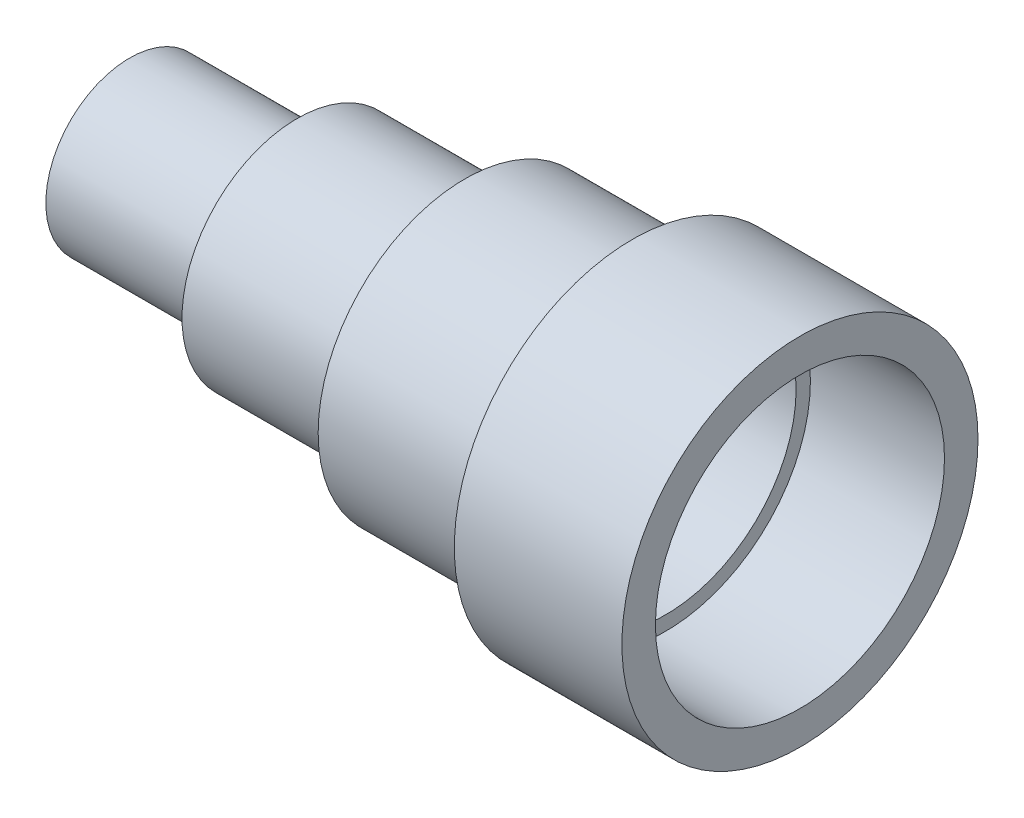
ISO-10303-21;
HEADER;
FILE_DESCRIPTION(('STEP AP214'),'2;1');
FILE_NAME('part.step','',(''),(''),'','','');
FILE_SCHEMA(('AUTOMOTIVE_DESIGN { 1 0 10303 214 1 1 1 1 }'));
ENDSEC;
DATA;
#1=APPLICATION_CONTEXT('core data for automotive mechanical design processes');
#2=APPLICATION_PROTOCOL_DEFINITION('international standard','automotive_design',2000,#1);
#3=PRODUCT_CONTEXT('',#1,'mechanical');
#4=PRODUCT('Part','Part','',(#3));
#5=PRODUCT_RELATED_PRODUCT_CATEGORY('part','',(#4));
#6=PRODUCT_DEFINITION_FORMATION('','',#4);
#7=PRODUCT_DEFINITION_CONTEXT('part definition',#1,'design');
#8=PRODUCT_DEFINITION('design','',#6,#7);
#9=PRODUCT_DEFINITION_SHAPE('','',#8);
#10=(LENGTH_UNIT() NAMED_UNIT(*) SI_UNIT(.MILLI.,.METRE.));
#11=(NAMED_UNIT(*) PLANE_ANGLE_UNIT() SI_UNIT($,.RADIAN.));
#12=(NAMED_UNIT(*) SI_UNIT($,.STERADIAN.) SOLID_ANGLE_UNIT());
#13=UNCERTAINTY_MEASURE_WITH_UNIT(LENGTH_MEASURE(1.E-05),#10,'distance_accuracy_value','');
#14=(GEOMETRIC_REPRESENTATION_CONTEXT(3) GLOBAL_UNCERTAINTY_ASSIGNED_CONTEXT((#13)) GLOBAL_UNIT_ASSIGNED_CONTEXT((#10,
#11,#12)) REPRESENTATION_CONTEXT('',''));
#15=CARTESIAN_POINT('',(0.,0.,0.));
#16=DIRECTION('',(0.,0.,1.));
#17=DIRECTION('',(1.,0.,0.));
#18=AXIS2_PLACEMENT_3D('',#15,#16,#17);
#19=CARTESIAN_POINT('',(40.,0.,-15.0355171036817));
#20=DIRECTION('',(1.,0.,0.));
#21=DIRECTION('',(0.,0.,-1.));
#22=AXIS2_PLACEMENT_3D('',#19,#20,#21);
#23=CYLINDRICAL_SURFACE('',#22,27.5);
#24=CARTESIAN_POINT('',(-40.,0.,-15.0355171036817));
#25=DIRECTION('',(1.,0.,0.));
#26=DIRECTION('',(0.,0.,-1.));
#27=AXIS2_PLACEMENT_3D('',#24,#25,#26);
#28=CIRCLE('',#27,27.5);
#29=CARTESIAN_POINT('',(-40.,0.,-42.5355171036817));
#30=VERTEX_POINT('',#29);
#31=EDGE_CURVE('E144',#30,#30,#28,.T.);
#32=ORIENTED_EDGE('',*,*,#31,.T.);
#33=EDGE_LOOP('',(#32));
#34=FACE_BOUND('',#33,.T.);
#35=CARTESIAN_POINT('',(0.,0.,-15.0355171036817));
#36=DIRECTION('',(1.,0.,0.));
#37=DIRECTION('',(0.,0.,-1.));
#38=AXIS2_PLACEMENT_3D('',#35,#36,#37);
#39=CIRCLE('',#38,27.5);
#40=CARTESIAN_POINT('',(0.,0.,-42.5355171036817));
#41=VERTEX_POINT('',#40);
#42=EDGE_CURVE('E102',#41,#41,#39,.T.);
#43=ORIENTED_EDGE('',*,*,#42,.F.);
#44=EDGE_LOOP('',(#43));
#45=FACE_BOUND('',#44,.T.);
#46=ADVANCED_FACE('F39',(#34,#45),#23,.T.);
#47=CARTESIAN_POINT('',(-40.,0.,-35.0355171036817));
#48=DIRECTION('',(-1.,0.,0.));
#49=DIRECTION('',(0.,0.,1.));
#50=AXIS2_PLACEMENT_3D('',#47,#48,#49);
#51=PLANE('',#50);
#52=CARTESIAN_POINT('',(-40.,0.,-15.0355171036817));
#53=DIRECTION('',(1.,0.,0.));
#54=DIRECTION('',(0.,0.,-1.));
#55=AXIS2_PLACEMENT_3D('',#52,#53,#54);
#56=CIRCLE('',#55,20.);
#57=CARTESIAN_POINT('',(-40.,0.,-35.0355171036817));
#58=VERTEX_POINT('',#57);
#59=EDGE_CURVE('E142',#58,#58,#56,.T.);
#60=ORIENTED_EDGE('',*,*,#59,.T.);
#61=EDGE_LOOP('',(#60));
#62=FACE_BOUND('',#61,.T.);
#63=ORIENTED_EDGE('',*,*,#31,.F.);
#64=EDGE_LOOP('',(#63));
#65=FACE_BOUND('',#64,.T.);
#66=ADVANCED_FACE('F175',(#62,#65),#51,.T.);
#67=CARTESIAN_POINT('',(40.,0.,-15.0355171036817));
#68=DIRECTION('',(1.,0.,0.));
#69=DIRECTION('',(0.,0.,-1.));
#70=AXIS2_PLACEMENT_3D('',#67,#68,#69);
#71=CYLINDRICAL_SURFACE('',#70,20.);
#72=CARTESIAN_POINT('',(-80.,0.,-15.0355171036817));
#73=DIRECTION('',(1.,0.,0.));
#74=DIRECTION('',(0.,0.,-1.));
#75=AXIS2_PLACEMENT_3D('',#72,#73,#74);
#76=CIRCLE('',#75,20.);
#77=CARTESIAN_POINT('',(-80.,0.,-35.0355171036817));
#78=VERTEX_POINT('',#77);
#79=EDGE_CURVE('E137',#78,#78,#76,.T.);
#80=ORIENTED_EDGE('',*,*,#79,.T.);
#81=EDGE_LOOP('',(#80));
#82=FACE_BOUND('',#81,.T.);
#83=ORIENTED_EDGE('',*,*,#59,.F.);
#84=EDGE_LOOP('',(#83));
#85=FACE_BOUND('',#84,.T.);
#86=ADVANCED_FACE('F176',(#82,#85),#71,.T.);
#87=CARTESIAN_POINT('',(-80.,0.,-15.0355171036817));
#88=DIRECTION('',(-1.,0.,0.));
#89=DIRECTION('',(0.,0.,1.));
#90=AXIS2_PLACEMENT_3D('',#87,#88,#89);
#91=PLANE('',#90);
#92=CARTESIAN_POINT('',(-80.,0.,-15.0355171036817));
#93=DIRECTION('',(-1.,0.,0.));
#94=DIRECTION('',(0.,0.,1.));
#95=AXIS2_PLACEMENT_3D('',#92,#93,#94);
#96=CIRCLE('',#95,15.);
#97=CARTESIAN_POINT('',(-80.,-14.6969384566991,-12.0355171036817));
#98=VERTEX_POINT('',#97);
#99=CARTESIAN_POINT('',(-80.,-14.6969384566991,-18.0355171036817));
#100=VERTEX_POINT('',#99);
#101=EDGE_CURVE('E52',#98,#100,#96,.T.);
#102=ORIENTED_EDGE('',*,*,#101,.F.);
#103=DIRECTION('',(0.,1.,0.));
#104=VECTOR('',#103,1.);
#105=CARTESIAN_POINT('',(-80.,-14.6969384566991,-12.0355171036817));
#106=LINE('',#105,#104);
#107=CARTESIAN_POINT('',(-80.,-18.,-12.0355171036817));
#108=VERTEX_POINT('',#107);
#109=EDGE_CURVE('E100',#108,#98,#106,.T.);
#110=ORIENTED_EDGE('',*,*,#109,.F.);
#111=DIRECTION('',(0.,0.,1.));
#112=VECTOR('',#111,1.);
#113=CARTESIAN_POINT('',(-80.,-18.,-15.0355171036817));
#114=LINE('',#113,#112);
#115=CARTESIAN_POINT('',(-80.,-18.,-18.0355171036817));
#116=VERTEX_POINT('',#115);
#117=EDGE_CURVE('E83',#116,#108,#114,.T.);
#118=ORIENTED_EDGE('',*,*,#117,.F.);
#119=DIRECTION('',(0.,-1.,0.));
#120=VECTOR('',#119,1.);
#121=CARTESIAN_POINT('',(-80.,-14.6969384566991,-18.0355171036817));
#122=LINE('',#121,#120);
#123=EDGE_CURVE('E89',#100,#116,#122,.T.);
#124=ORIENTED_EDGE('',*,*,#123,.F.);
#125=EDGE_LOOP('',(#102,#110,#118,#124));
#126=FACE_BOUND('',#125,.T.);
#127=ORIENTED_EDGE('',*,*,#79,.F.);
#128=EDGE_LOOP('',(#127));
#129=FACE_BOUND('',#128,.T.);
#130=ADVANCED_FACE('F94',(#126,#129),#91,.T.);
#131=CARTESIAN_POINT('',(-32.,0.,-40.273612341777));
#132=DIRECTION('',(1.,0.,0.));
#133=DIRECTION('',(0.,0.,-1.));
#134=AXIS2_PLACEMENT_3D('',#131,#132,#133);
#135=PLANE('',#134);
#136=CARTESIAN_POINT('',(-32.,0.,-15.0355171036817));
#137=DIRECTION('',(1.,0.,0.));
#138=DIRECTION('',(0.,0.,-1.));
#139=AXIS2_PLACEMENT_3D('',#136,#137,#138);
#140=CIRCLE('',#139,15.);
#141=CARTESIAN_POINT('',(-32.,-14.6969384566991,-18.0355171036817));
#142=VERTEX_POINT('',#141);
#143=CARTESIAN_POINT('',(-32.,-14.6969384566991,-12.0355171036817));
#144=VERTEX_POINT('',#143);
#145=EDGE_CURVE('E11',#142,#144,#140,.T.);
#146=ORIENTED_EDGE('',*,*,#145,.F.);
#147=DIRECTION('',(0.,1.,0.));
#148=VECTOR('',#147,1.);
#149=CARTESIAN_POINT('',(-32.,0.,-18.0355171036817));
#150=LINE('',#149,#148);
#151=CARTESIAN_POINT('',(-32.,-18.,-18.0355171036817));
#152=VERTEX_POINT('',#151);
#153=EDGE_CURVE('E146',#152,#142,#150,.T.);
#154=ORIENTED_EDGE('',*,*,#153,.F.);
#155=DIRECTION('',(0.,0.,-1.));
#156=VECTOR('',#155,1.);
#157=CARTESIAN_POINT('',(-32.,-18.,-40.273612341777));
#158=LINE('',#157,#156);
#159=CARTESIAN_POINT('',(-32.,-18.,-12.0355171036817));
#160=VERTEX_POINT('',#159);
#161=EDGE_CURVE('E82',#160,#152,#158,.T.);
#162=ORIENTED_EDGE('',*,*,#161,.F.);
#163=DIRECTION('',(0.,-1.,0.));
#164=VECTOR('',#163,1.);
#165=CARTESIAN_POINT('',(-32.,0.,-12.0355171036817));
#166=LINE('',#165,#164);
#167=EDGE_CURVE('E46',#144,#160,#166,.T.);
#168=ORIENTED_EDGE('',*,*,#167,.F.);
#169=EDGE_LOOP('',(#146,#154,#162,#168));
#170=FACE_BOUND('',#169,.T.);
#171=CARTESIAN_POINT('',(-32.,0.,-15.0355171036817));
#172=DIRECTION('',(1.,0.,0.));
#173=DIRECTION('',(0.,0.,-1.));
#174=AXIS2_PLACEMENT_3D('',#171,#172,#173);
#175=CIRCLE('',#174,25.2380952380952);
#176=CARTESIAN_POINT('',(-32.,0.,-40.273612341777));
#177=VERTEX_POINT('',#176);
#178=EDGE_CURVE('E138',#177,#177,#175,.T.);
#179=ORIENTED_EDGE('',*,*,#178,.T.);
#180=EDGE_LOOP('',(#179));
#181=FACE_BOUND('',#180,.T.);
#182=ADVANCED_FACE('F156',(#170,#181),#135,.T.);
#183=CARTESIAN_POINT('',(40.,0.,-15.0355171036817));
#184=DIRECTION('',(1.,0.,0.));
#185=DIRECTION('',(0.,0.,-1.));
#186=AXIS2_PLACEMENT_3D('',#183,#184,#185);
#187=CYLINDRICAL_SURFACE('',#186,25.2380952380952);
#188=CARTESIAN_POINT('',(8.00000000000001,0.,-15.0355171036817));
#189=DIRECTION('',(1.,0.,0.));
#190=DIRECTION('',(0.,0.,-1.));
#191=AXIS2_PLACEMENT_3D('',#188,#189,#190);
#192=CIRCLE('',#191,25.2380952380952);
#193=CARTESIAN_POINT('',(8.,0.,-40.273612341777));
#194=VERTEX_POINT('',#193);
#195=EDGE_CURVE('E135',#194,#194,#192,.T.);
#196=ORIENTED_EDGE('',*,*,#195,.T.);
#197=EDGE_LOOP('',(#196));
#198=FACE_BOUND('',#197,.T.);
#199=ORIENTED_EDGE('',*,*,#178,.F.);
#200=EDGE_LOOP('',(#199));
#201=FACE_BOUND('',#200,.T.);
#202=ADVANCED_FACE('F227',(#198,#201),#187,.F.);
#203=CARTESIAN_POINT('',(8.,0.,-46.1228186909833));
#204=DIRECTION('',(1.,0.,0.));
#205=DIRECTION('',(0.,0.,-1.));
#206=AXIS2_PLACEMENT_3D('',#203,#204,#205);
#207=PLANE('',#206);
#208=CARTESIAN_POINT('',(8.00000000000001,0.,-15.0355171036817));
#209=DIRECTION('',(1.,0.,0.));
#210=DIRECTION('',(0.,0.,-1.));
#211=AXIS2_PLACEMENT_3D('',#208,#209,#210);
#212=CIRCLE('',#211,31.0873015873016);
#213=CARTESIAN_POINT('',(8.00000000000001,0.,-46.1228186909833));
#214=VERTEX_POINT('',#213);
#215=EDGE_CURVE('E128',#214,#214,#212,.T.);
#216=ORIENTED_EDGE('',*,*,#215,.T.);
#217=EDGE_LOOP('',(#216));
#218=FACE_BOUND('',#217,.T.);
#219=ORIENTED_EDGE('',*,*,#195,.F.);
#220=EDGE_LOOP('',(#219));
#221=FACE_BOUND('',#220,.T.);
#222=ADVANCED_FACE('F221',(#218,#221),#207,.T.);
#223=CARTESIAN_POINT('',(40.,0.,-15.0355171036817));
#224=DIRECTION('',(1.,0.,0.));
#225=DIRECTION('',(0.,0.,-1.));
#226=AXIS2_PLACEMENT_3D('',#223,#224,#225);
#227=CYLINDRICAL_SURFACE('',#226,31.0873015873016);
#228=CARTESIAN_POINT('',(48.,0.,-15.0355171036817));
#229=DIRECTION('',(1.,0.,0.));
#230=DIRECTION('',(0.,0.,-1.));
#231=AXIS2_PLACEMENT_3D('',#228,#229,#230);
#232=CIRCLE('',#231,31.0873015873016);
#233=CARTESIAN_POINT('',(48.,0.,-46.1228186909833));
#234=VERTEX_POINT('',#233);
#235=EDGE_CURVE('E130',#234,#234,#232,.T.);
#236=ORIENTED_EDGE('',*,*,#235,.T.);
#237=EDGE_LOOP('',(#236));
#238=FACE_BOUND('',#237,.T.);
#239=ORIENTED_EDGE('',*,*,#215,.F.);
#240=EDGE_LOOP('',(#239));
#241=FACE_BOUND('',#240,.T.);
#242=ADVANCED_FACE('F217',(#238,#241),#227,.F.);
#243=CARTESIAN_POINT('',(48.,0.,-49.5355171036817));
#244=DIRECTION('',(1.,0.,0.));
#245=DIRECTION('',(0.,0.,-1.));
#246=AXIS2_PLACEMENT_3D('',#243,#244,#245);
#247=PLANE('',#246);
#248=CARTESIAN_POINT('',(48.,0.,-15.0355171036817));
#249=DIRECTION('',(1.,0.,0.));
#250=DIRECTION('',(0.,0.,-1.));
#251=AXIS2_PLACEMENT_3D('',#248,#249,#250);
#252=CIRCLE('',#251,34.5);
#253=CARTESIAN_POINT('',(48.,0.,-49.5355171036817));
#254=VERTEX_POINT('',#253);
#255=EDGE_CURVE('E122',#254,#254,#252,.T.);
#256=ORIENTED_EDGE('',*,*,#255,.T.);
#257=EDGE_LOOP('',(#256));
#258=FACE_BOUND('',#257,.T.);
#259=ORIENTED_EDGE('',*,*,#235,.F.);
#260=EDGE_LOOP('',(#259));
#261=FACE_BOUND('',#260,.T.);
#262=ADVANCED_FACE('F215',(#258,#261),#247,.T.);
#263=CARTESIAN_POINT('',(40.,0.,-15.0355171036817));
#264=DIRECTION('',(1.,0.,0.));
#265=DIRECTION('',(0.,0.,-1.));
#266=AXIS2_PLACEMENT_3D('',#263,#264,#265);
#267=CYLINDRICAL_SURFACE('',#266,34.5);
#268=CARTESIAN_POINT('',(80.,0.,-15.0355171036817));
#269=DIRECTION('',(1.,0.,0.));
#270=DIRECTION('',(0.,0.,-1.));
#271=AXIS2_PLACEMENT_3D('',#268,#269,#270);
#272=CIRCLE('',#271,34.5);
#273=CARTESIAN_POINT('',(80.,0.,-49.5355171036817));
#274=VERTEX_POINT('',#273);
#275=EDGE_CURVE('E123',#274,#274,#272,.T.);
#276=ORIENTED_EDGE('',*,*,#275,.T.);
#277=EDGE_LOOP('',(#276));
#278=FACE_BOUND('',#277,.T.);
#279=ORIENTED_EDGE('',*,*,#255,.F.);
#280=EDGE_LOOP('',(#279));
#281=FACE_BOUND('',#280,.T.);
#282=ADVANCED_FACE('F206',(#278,#281),#267,.F.);
#283=CARTESIAN_POINT('',(80.,0.,-57.5355171036817));
#284=DIRECTION('',(1.,0.,0.));
#285=DIRECTION('',(0.,0.,-1.));
#286=AXIS2_PLACEMENT_3D('',#283,#284,#285);
#287=PLANE('',#286);
#288=CARTESIAN_POINT('',(80.,0.,-15.0355171036817));
#289=DIRECTION('',(1.,0.,0.));
#290=DIRECTION('',(0.,0.,-1.));
#291=AXIS2_PLACEMENT_3D('',#288,#289,#290);
#292=CIRCLE('',#291,42.5);
#293=CARTESIAN_POINT('',(80.,0.,-57.5355171036817));
#294=VERTEX_POINT('',#293);
#295=EDGE_CURVE('E120',#294,#294,#292,.T.);
#296=ORIENTED_EDGE('',*,*,#295,.T.);
#297=EDGE_LOOP('',(#296));
#298=FACE_BOUND('',#297,.T.);
#299=ORIENTED_EDGE('',*,*,#275,.F.);
#300=EDGE_LOOP('',(#299));
#301=FACE_BOUND('',#300,.T.);
#302=ADVANCED_FACE('F199',(#298,#301),#287,.T.);
#303=CARTESIAN_POINT('',(40.,0.,-15.0355171036817));
#304=DIRECTION('',(1.,0.,0.));
#305=DIRECTION('',(0.,0.,-1.));
#306=AXIS2_PLACEMENT_3D('',#303,#304,#305);
#307=CYLINDRICAL_SURFACE('',#306,42.5);
#308=CARTESIAN_POINT('',(40.,0.,-15.0355171036817));
#309=DIRECTION('',(1.,0.,0.));
#310=DIRECTION('',(0.,0.,-1.));
#311=AXIS2_PLACEMENT_3D('',#308,#309,#310);
#312=CIRCLE('',#311,42.5);
#313=CARTESIAN_POINT('',(40.,0.,-57.5355171036817));
#314=VERTEX_POINT('',#313);
#315=EDGE_CURVE('E113',#314,#314,#312,.T.);
#316=ORIENTED_EDGE('',*,*,#315,.T.);
#317=EDGE_LOOP('',(#316));
#318=FACE_BOUND('',#317,.T.);
#319=ORIENTED_EDGE('',*,*,#295,.F.);
#320=EDGE_LOOP('',(#319));
#321=FACE_BOUND('',#320,.T.);
#322=ADVANCED_FACE('F192',(#318,#321),#307,.T.);
#323=CARTESIAN_POINT('',(40.,0.,-50.0355171036817));
#324=DIRECTION('',(-1.,0.,0.));
#325=DIRECTION('',(0.,0.,1.));
#326=AXIS2_PLACEMENT_3D('',#323,#324,#325);
#327=PLANE('',#326);
#328=CARTESIAN_POINT('',(40.,0.,-15.0355171036817));
#329=DIRECTION('',(1.,0.,0.));
#330=DIRECTION('',(0.,0.,-1.));
#331=AXIS2_PLACEMENT_3D('',#328,#329,#330);
#332=CIRCLE('',#331,35.);
#333=CARTESIAN_POINT('',(40.,0.,-50.0355171036817));
#334=VERTEX_POINT('',#333);
#335=EDGE_CURVE('E115',#334,#334,#332,.T.);
#336=ORIENTED_EDGE('',*,*,#335,.T.);
#337=EDGE_LOOP('',(#336));
#338=FACE_BOUND('',#337,.T.);
#339=ORIENTED_EDGE('',*,*,#315,.F.);
#340=EDGE_LOOP('',(#339));
#341=FACE_BOUND('',#340,.T.);
#342=ADVANCED_FACE('F190',(#338,#341),#327,.T.);
#343=CARTESIAN_POINT('',(40.,0.,-15.0355171036817));
#344=DIRECTION('',(1.,0.,0.));
#345=DIRECTION('',(0.,0.,-1.));
#346=AXIS2_PLACEMENT_3D('',#343,#344,#345);
#347=CYLINDRICAL_SURFACE('',#346,35.);
#348=CARTESIAN_POINT('',(0.,0.,-15.0355171036817));
#349=DIRECTION('',(1.,0.,0.));
#350=DIRECTION('',(0.,0.,-1.));
#351=AXIS2_PLACEMENT_3D('',#348,#349,#350);
#352=CIRCLE('',#351,35.);
#353=CARTESIAN_POINT('',(0.,0.,-50.0355171036817));
#354=VERTEX_POINT('',#353);
#355=EDGE_CURVE('E108',#354,#354,#352,.T.);
#356=ORIENTED_EDGE('',*,*,#355,.T.);
#357=EDGE_LOOP('',(#356));
#358=FACE_BOUND('',#357,.T.);
#359=ORIENTED_EDGE('',*,*,#335,.F.);
#360=EDGE_LOOP('',(#359));
#361=FACE_BOUND('',#360,.T.);
#362=ADVANCED_FACE('F169',(#358,#361),#347,.T.);
#363=CARTESIAN_POINT('',(0.,0.,-42.5355171036817));
#364=DIRECTION('',(-1.,0.,0.));
#365=DIRECTION('',(0.,0.,1.));
#366=AXIS2_PLACEMENT_3D('',#363,#364,#365);
#367=PLANE('',#366);
#368=ORIENTED_EDGE('',*,*,#42,.T.);
#369=EDGE_LOOP('',(#368));
#370=FACE_BOUND('',#369,.T.);
#371=ORIENTED_EDGE('',*,*,#355,.F.);
#372=EDGE_LOOP('',(#371));
#373=FACE_BOUND('',#372,.T.);
#374=ADVANCED_FACE('F159',(#370,#373),#367,.T.);
#375=CARTESIAN_POINT('',(80.,0.,-15.0355171036817));
#376=DIRECTION('',(-1.,0.,0.));
#377=DIRECTION('',(0.,0.,1.));
#378=AXIS2_PLACEMENT_3D('',#375,#376,#377);
#379=CYLINDRICAL_SURFACE('',#378,15.);
#380=ORIENTED_EDGE('',*,*,#145,.T.);
#381=DIRECTION('',(-1.,0.,0.));
#382=VECTOR('',#381,1.);
#383=CARTESIAN_POINT('',(80.,-14.6969384566991,-12.0355171036817));
#384=LINE('',#383,#382);
#385=EDGE_CURVE('E105',#144,#98,#384,.T.);
#386=ORIENTED_EDGE('',*,*,#385,.T.);
#387=ORIENTED_EDGE('',*,*,#101,.T.);
#388=DIRECTION('',(-1.,0.,0.));
#389=VECTOR('',#388,1.);
#390=CARTESIAN_POINT('',(80.,-14.6969384566991,-18.0355171036818));
#391=LINE('',#390,#389);
#392=EDGE_CURVE('E87',#142,#100,#391,.T.);
#393=ORIENTED_EDGE('',*,*,#392,.F.);
#394=EDGE_LOOP('',(#380,#386,#387,#393));
#395=FACE_BOUND('',#394,.T.);
#396=ADVANCED_FACE('F158',(#395),#379,.F.);
#397=CARTESIAN_POINT('',(80.,-14.6969384566991,-12.0355171036817));
#398=DIRECTION('',(0.,0.,1.));
#399=DIRECTION('',(1.,0.,0.));
#400=AXIS2_PLACEMENT_3D('',#397,#398,#399);
#401=PLANE('',#400);
#402=ORIENTED_EDGE('',*,*,#167,.T.);
#403=DIRECTION('',(-1.,0.,0.));
#404=VECTOR('',#403,1.);
#405=CARTESIAN_POINT('',(80.,-18.,-12.0355171036817));
#406=LINE('',#405,#404);
#407=EDGE_CURVE('E88',#160,#108,#406,.T.);
#408=ORIENTED_EDGE('',*,*,#407,.T.);
#409=ORIENTED_EDGE('',*,*,#109,.T.);
#410=ORIENTED_EDGE('',*,*,#385,.F.);
#411=EDGE_LOOP('',(#402,#408,#409,#410));
#412=FACE_BOUND('',#411,.T.);
#413=ADVANCED_FACE('F153',(#412),#401,.F.);
#414=CARTESIAN_POINT('',(80.,-18.,-15.0355171036817));
#415=DIRECTION('',(0.,-1.,0.));
#416=DIRECTION('',(0.,0.,-1.));
#417=AXIS2_PLACEMENT_3D('',#414,#415,#416);
#418=PLANE('',#417);
#419=ORIENTED_EDGE('',*,*,#161,.T.);
#420=DIRECTION('',(-1.,0.,0.));
#421=VECTOR('',#420,1.);
#422=CARTESIAN_POINT('',(80.,-18.,-18.0355171036818));
#423=LINE('',#422,#421);
#424=EDGE_CURVE('E64',#152,#116,#423,.T.);
#425=ORIENTED_EDGE('',*,*,#424,.T.);
#426=ORIENTED_EDGE('',*,*,#117,.T.);
#427=ORIENTED_EDGE('',*,*,#407,.F.);
#428=EDGE_LOOP('',(#419,#425,#426,#427));
#429=FACE_BOUND('',#428,.T.);
#430=ADVANCED_FACE('F80',(#429),#418,.F.);
#431=CARTESIAN_POINT('',(80.,-14.6969384566991,-18.0355171036818));
#432=DIRECTION('',(0.,0.,-1.));
#433=DIRECTION('',(-1.,0.,0.));
#434=AXIS2_PLACEMENT_3D('',#431,#432,#433);
#435=PLANE('',#434);
#436=ORIENTED_EDGE('',*,*,#153,.T.);
#437=ORIENTED_EDGE('',*,*,#392,.T.);
#438=ORIENTED_EDGE('',*,*,#123,.T.);
#439=ORIENTED_EDGE('',*,*,#424,.F.);
#440=EDGE_LOOP('',(#436,#437,#438,#439));
#441=FACE_BOUND('',#440,.T.);
#442=ADVANCED_FACE('F93',(#441),#435,.F.);
#443=CLOSED_SHELL('',(#46,#66,#86,#130,#182,#202,#222,#242,#262,#282,#302,#322,#342,#362,#374,
#396,#413,#430,#442));
#444=MANIFOLD_SOLID_BREP('B2',#443);
#445=ADVANCED_BREP_SHAPE_REPRESENTATION('',(#18,#444),#14);
#446=SHAPE_DEFINITION_REPRESENTATION(#9,#445);
ENDSEC;
END-ISO-10303-21;
